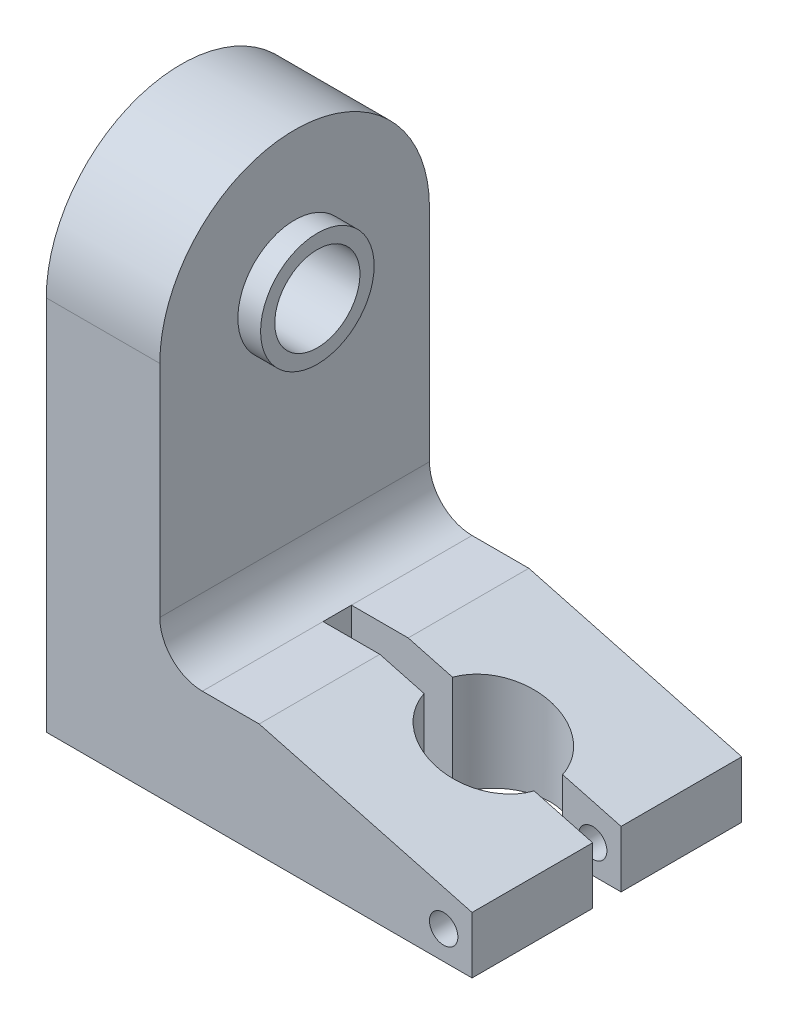
ISO-10303-21;
HEADER;
FILE_DESCRIPTION(('STEP AP214'),'2;1');
FILE_NAME('part.step','',(''),(''),'','','');
FILE_SCHEMA(('AUTOMOTIVE_DESIGN { 1 0 10303 214 1 1 1 1 }'));
ENDSEC;
DATA;
#1=APPLICATION_CONTEXT('core data for automotive mechanical design processes');
#2=APPLICATION_PROTOCOL_DEFINITION('international standard','automotive_design',2000,#1);
#3=PRODUCT_CONTEXT('',#1,'mechanical');
#4=PRODUCT('Part','Part','',(#3));
#5=PRODUCT_RELATED_PRODUCT_CATEGORY('part','',(#4));
#6=PRODUCT_DEFINITION_FORMATION('','',#4);
#7=PRODUCT_DEFINITION_CONTEXT('part definition',#1,'design');
#8=PRODUCT_DEFINITION('design','',#6,#7);
#9=PRODUCT_DEFINITION_SHAPE('','',#8);
#10=(LENGTH_UNIT() NAMED_UNIT(*) SI_UNIT(.MILLI.,.METRE.));
#11=(NAMED_UNIT(*) PLANE_ANGLE_UNIT() SI_UNIT($,.RADIAN.));
#12=(NAMED_UNIT(*) SI_UNIT($,.STERADIAN.) SOLID_ANGLE_UNIT());
#13=UNCERTAINTY_MEASURE_WITH_UNIT(LENGTH_MEASURE(1.E-05),#10,'distance_accuracy_value','');
#14=(GEOMETRIC_REPRESENTATION_CONTEXT(3) GLOBAL_UNCERTAINTY_ASSIGNED_CONTEXT((#13)) GLOBAL_UNIT_ASSIGNED_CONTEXT((#10,
#11,#12)) REPRESENTATION_CONTEXT('',''));
#15=CARTESIAN_POINT('',(0.,0.,0.));
#16=DIRECTION('',(0.,0.,1.));
#17=DIRECTION('',(1.,0.,0.));
#18=AXIS2_PLACEMENT_3D('',#15,#16,#17);
#19=CARTESIAN_POINT('',(150.,0.,47.5));
#20=DIRECTION('',(-1.,0.,0.));
#21=DIRECTION('',(0.,0.,1.));
#22=AXIS2_PLACEMENT_3D('',#19,#20,#21);
#23=PLANE('',#22);
#24=DIRECTION('',(0.,0.,-1.));
#25=VECTOR('',#24,1.);
#26=CARTESIAN_POINT('',(150.,20.,47.5));
#27=LINE('',#26,#25);
#28=CARTESIAN_POINT('',(150.,20.,-5.));
#29=VERTEX_POINT('',#28);
#30=CARTESIAN_POINT('',(150.,20.,-47.5));
#31=VERTEX_POINT('',#30);
#32=EDGE_CURVE('E168',#29,#31,#27,.T.);
#33=ORIENTED_EDGE('',*,*,#32,.F.);
#34=DIRECTION('',(0.,1.,0.));
#35=VECTOR('',#34,1.);
#36=CARTESIAN_POINT('',(150.,-25.,-5.));
#37=LINE('',#36,#35);
#38=CARTESIAN_POINT('',(150.,0.,-5.));
#39=VERTEX_POINT('',#38);
#40=EDGE_CURVE('E226',#39,#29,#37,.T.);
#41=ORIENTED_EDGE('',*,*,#40,.F.);
#42=DIRECTION('',(0.,0.,-1.));
#43=VECTOR('',#42,1.);
#44=CARTESIAN_POINT('',(150.,0.,47.5));
#45=LINE('',#44,#43);
#46=CARTESIAN_POINT('',(150.,0.,-47.5));
#47=VERTEX_POINT('',#46);
#48=EDGE_CURVE('E173',#39,#47,#45,.T.);
#49=ORIENTED_EDGE('',*,*,#48,.T.);
#50=DIRECTION('',(0.,1.,0.));
#51=VECTOR('',#50,1.);
#52=CARTESIAN_POINT('',(150.,0.,-47.5));
#53=LINE('',#52,#51);
#54=EDGE_CURVE('E149',#47,#31,#53,.T.);
#55=ORIENTED_EDGE('',*,*,#54,.T.);
#56=EDGE_LOOP('',(#33,#41,#49,#55));
#57=FACE_BOUND('',#56,.T.);
#58=ADVANCED_FACE('F39',(#57),#23,.F.);
#59=CARTESIAN_POINT('',(150.,20.,47.5));
#60=DIRECTION('',(-0.257662650560332,-0.966234939601246,0.));
#61=DIRECTION('',(0.966234939601246,-0.257662650560332,0.));
#62=AXIS2_PLACEMENT_3D('',#59,#60,#61);
#63=PLANE('',#62);
#64=CARTESIAN_POINT('',(150.,20.,47.5));
#65=VERTEX_POINT('',#64);
#66=CARTESIAN_POINT('',(150.,20.,5.));
#67=VERTEX_POINT('',#66);
#68=EDGE_CURVE('E171',#65,#67,#27,.T.);
#69=ORIENTED_EDGE('',*,*,#68,.T.);
#70=DIRECTION('',(-0.966234939601246,0.257662650560332,0.));
#71=VECTOR('',#70,1.);
#72=CARTESIAN_POINT('',(150.,20.,5.));
#73=LINE('',#72,#71);
#74=CARTESIAN_POINT('',(129.364916731037,25.5026888717234,5.));
#75=VERTEX_POINT('',#74);
#76=EDGE_CURVE('E11',#67,#75,#73,.T.);
#77=ORIENTED_EDGE('',*,*,#76,.T.);
#78=CARTESIAN_POINT('',(110.,30.6666666666667,0.));
#79=DIRECTION('',(-0.257662650560332,-0.966234939601246,0.));
#80=DIRECTION('',(-0.966234939601246,0.257662650560332,0.));
#81=AXIS2_PLACEMENT_3D('',#78,#79,#80);
#82=ELLIPSE('',#81,20.6988995950134,20.);
#83=CARTESIAN_POINT('',(90.6350832689629,35.8306444616099,5.));
#84=VERTEX_POINT('',#83);
#85=EDGE_CURVE('E48',#75,#84,#82,.T.);
#86=ORIENTED_EDGE('',*,*,#85,.T.);
#87=DIRECTION('',(-0.966234939601246,0.257662650560332,0.));
#88=VECTOR('',#87,1.);
#89=CARTESIAN_POINT('',(150.,20.,5.00000000000001));
#90=LINE('',#89,#88);
#91=CARTESIAN_POINT('',(75.,40.,5.));
#92=VERTEX_POINT('',#91);
#93=EDGE_CURVE('E196',#84,#92,#90,.T.);
#94=ORIENTED_EDGE('',*,*,#93,.T.);
#95=DIRECTION('',(0.,0.,-1.));
#96=VECTOR('',#95,1.);
#97=CARTESIAN_POINT('',(75.,40.,47.5));
#98=LINE('',#97,#96);
#99=CARTESIAN_POINT('',(75.,40.,47.5));
#100=VERTEX_POINT('',#99);
#101=EDGE_CURVE('E170',#100,#92,#98,.T.);
#102=ORIENTED_EDGE('',*,*,#101,.F.);
#103=DIRECTION('',(-0.966234939601246,0.257662650560332,0.));
#104=VECTOR('',#103,1.);
#105=CARTESIAN_POINT('',(150.,20.,47.5));
#106=LINE('',#105,#104);
#107=EDGE_CURVE('E278',#65,#100,#106,.T.);
#108=ORIENTED_EDGE('',*,*,#107,.F.);
#109=EDGE_LOOP('',(#69,#77,#86,#94,#102,#108));
#110=FACE_BOUND('',#109,.T.);
#111=ADVANCED_FACE('F195',(#110),#63,.F.);
#112=CARTESIAN_POINT('',(75.,40.,47.5));
#113=DIRECTION('',(0.,-1.,0.));
#114=DIRECTION('',(1.,0.,0.));
#115=AXIS2_PLACEMENT_3D('',#112,#113,#114);
#116=PLANE('',#115);
#117=ORIENTED_EDGE('',*,*,#101,.T.);
#118=DIRECTION('',(1.,0.,0.));
#119=VECTOR('',#118,1.);
#120=CARTESIAN_POINT('',(55.0000000000001,40.,5.));
#121=LINE('',#120,#119);
#122=CARTESIAN_POINT('',(55.0000000000001,40.,5.));
#123=VERTEX_POINT('',#122);
#124=EDGE_CURVE('E239',#123,#92,#121,.T.);
#125=ORIENTED_EDGE('',*,*,#124,.F.);
#126=DIRECTION('',(0.,0.,-1.));
#127=VECTOR('',#126,1.);
#128=CARTESIAN_POINT('',(55.0000000000001,40.,47.5));
#129=LINE('',#128,#127);
#130=CARTESIAN_POINT('',(55.0000000000001,40.,47.5));
#131=VERTEX_POINT('',#130);
#132=EDGE_CURVE('E163',#131,#123,#129,.T.);
#133=ORIENTED_EDGE('',*,*,#132,.F.);
#134=DIRECTION('',(-1.,0.,0.));
#135=VECTOR('',#134,1.);
#136=CARTESIAN_POINT('',(75.,40.,47.5));
#137=LINE('',#136,#135);
#138=EDGE_CURVE('E121',#100,#131,#137,.T.);
#139=ORIENTED_EDGE('',*,*,#138,.F.);
#140=EDGE_LOOP('',(#117,#125,#133,#139));
#141=FACE_BOUND('',#140,.T.);
#142=ADVANCED_FACE('F288',(#141),#116,.F.);
#143=CARTESIAN_POINT('',(0.,0.,47.5));
#144=DIRECTION('',(1.,0.,0.));
#145=DIRECTION('',(0.,0.,-1.));
#146=AXIS2_PLACEMENT_3D('',#143,#144,#145);
#147=PLANE('',#146);
#148=CARTESIAN_POINT('',(0.,132.5,0.));
#149=DIRECTION('',(1.,0.,0.));
#150=DIRECTION('',(0.,0.,-1.));
#151=AXIS2_PLACEMENT_3D('',#148,#149,#150);
#152=CIRCLE('',#151,15.);
#153=CARTESIAN_POINT('',(0.,132.5,-15.));
#154=VERTEX_POINT('',#153);
#155=EDGE_CURVE('E266',#154,#154,#152,.T.);
#156=ORIENTED_EDGE('',*,*,#155,.T.);
#157=EDGE_LOOP('',(#156));
#158=FACE_BOUND('',#157,.T.);
#159=DIRECTION('',(0.,-1.,0.));
#160=VECTOR('',#159,1.);
#161=CARTESIAN_POINT('',(0.,0.,-47.5));
#162=LINE('',#161,#160);
#163=CARTESIAN_POINT('',(0.,132.5,-47.5));
#164=VERTEX_POINT('',#163);
#165=CARTESIAN_POINT('',(0.,0.,-47.5));
#166=VERTEX_POINT('',#165);
#167=EDGE_CURVE('E141',#164,#166,#162,.T.);
#168=ORIENTED_EDGE('',*,*,#167,.T.);
#169=DIRECTION('',(0.,0.,-1.));
#170=VECTOR('',#169,1.);
#171=CARTESIAN_POINT('',(0.,0.,47.5));
#172=LINE('',#171,#170);
#173=CARTESIAN_POINT('',(0.,0.,47.5));
#174=VERTEX_POINT('',#173);
#175=EDGE_CURVE('E177',#174,#166,#172,.T.);
#176=ORIENTED_EDGE('',*,*,#175,.F.);
#177=DIRECTION('',(0.,-1.,0.));
#178=VECTOR('',#177,1.);
#179=CARTESIAN_POINT('',(0.,0.,47.5));
#180=LINE('',#179,#178);
#181=CARTESIAN_POINT('',(0.,132.5,47.5));
#182=VERTEX_POINT('',#181);
#183=EDGE_CURVE('E165',#182,#174,#180,.T.);
#184=ORIENTED_EDGE('',*,*,#183,.F.);
#185=CARTESIAN_POINT('',(0.,132.5,0.));
#186=DIRECTION('',(-1.,0.,0.));
#187=DIRECTION('',(0.,0.,1.));
#188=AXIS2_PLACEMENT_3D('',#185,#186,#187);
#189=CIRCLE('',#188,47.5);
#190=EDGE_CURVE('E275',#182,#164,#189,.T.);
#191=ORIENTED_EDGE('',*,*,#190,.T.);
#192=EDGE_LOOP('',(#168,#176,#184,#191));
#193=FACE_BOUND('',#192,.T.);
#194=ADVANCED_FACE('F41',(#158,#193),#147,.F.);
#195=CARTESIAN_POINT('',(0.,0.,47.5));
#196=DIRECTION('',(0.,1.,0.));
#197=DIRECTION('',(0.,0.,1.));
#198=AXIS2_PLACEMENT_3D('',#195,#196,#197);
#199=PLANE('',#198);
#200=ORIENTED_EDGE('',*,*,#48,.F.);
#201=DIRECTION('',(-1.,0.,0.));
#202=VECTOR('',#201,1.);
#203=CARTESIAN_POINT('',(0.,0.,-4.99999999999991));
#204=LINE('',#203,#202);
#205=CARTESIAN_POINT('',(129.364916731037,0.,-4.99999999999999));
#206=VERTEX_POINT('',#205);
#207=EDGE_CURVE('E260',#39,#206,#204,.T.);
#208=ORIENTED_EDGE('',*,*,#207,.T.);
#209=CARTESIAN_POINT('',(110.,0.,0.));
#210=DIRECTION('',(0.,1.,0.));
#211=DIRECTION('',(0.,0.,1.));
#212=AXIS2_PLACEMENT_3D('',#209,#210,#211);
#213=CIRCLE('',#212,20.);
#214=CARTESIAN_POINT('',(90.6350832689629,0.,-4.99999999999998));
#215=VERTEX_POINT('',#214);
#216=EDGE_CURVE('E257',#206,#215,#213,.T.);
#217=ORIENTED_EDGE('',*,*,#216,.T.);
#218=DIRECTION('',(-1.,0.,0.));
#219=VECTOR('',#218,1.);
#220=CARTESIAN_POINT('',(0.,0.,-5.00000000000002));
#221=LINE('',#220,#219);
#222=CARTESIAN_POINT('',(55.0000000000001,0.,-5.));
#223=VERTEX_POINT('',#222);
#224=EDGE_CURVE('E249',#215,#223,#221,.T.);
#225=ORIENTED_EDGE('',*,*,#224,.T.);
#226=DIRECTION('',(0.,0.,1.));
#227=VECTOR('',#226,1.);
#228=CARTESIAN_POINT('',(55.0000000000001,0.,47.5));
#229=LINE('',#228,#227);
#230=CARTESIAN_POINT('',(55.0000000000001,0.,5.));
#231=VERTEX_POINT('',#230);
#232=EDGE_CURVE('E238',#223,#231,#229,.T.);
#233=ORIENTED_EDGE('',*,*,#232,.T.);
#234=DIRECTION('',(1.,0.,0.));
#235=VECTOR('',#234,1.);
#236=CARTESIAN_POINT('',(0.,0.,4.99999999999999));
#237=LINE('',#236,#235);
#238=CARTESIAN_POINT('',(90.6350832689629,0.,5.));
#239=VERTEX_POINT('',#238);
#240=EDGE_CURVE('E253',#231,#239,#237,.T.);
#241=ORIENTED_EDGE('',*,*,#240,.T.);
#242=CARTESIAN_POINT('',(110.,0.,0.));
#243=DIRECTION('',(0.,1.,0.));
#244=DIRECTION('',(0.,0.,1.));
#245=AXIS2_PLACEMENT_3D('',#242,#243,#244);
#246=CIRCLE('',#245,20.);
#247=CARTESIAN_POINT('',(129.364916731037,0.,5.));
#248=VERTEX_POINT('',#247);
#249=EDGE_CURVE('E255',#239,#248,#246,.T.);
#250=ORIENTED_EDGE('',*,*,#249,.T.);
#251=DIRECTION('',(1.,0.,0.));
#252=VECTOR('',#251,1.);
#253=CARTESIAN_POINT('',(0.,0.,5.00000000000002));
#254=LINE('',#253,#252);
#255=CARTESIAN_POINT('',(150.,0.,5.));
#256=VERTEX_POINT('',#255);
#257=EDGE_CURVE('E224',#248,#256,#254,.T.);
#258=ORIENTED_EDGE('',*,*,#257,.T.);
#259=CARTESIAN_POINT('',(150.,0.,47.5));
#260=VERTEX_POINT('',#259);
#261=EDGE_CURVE('E175',#260,#256,#45,.T.);
#262=ORIENTED_EDGE('',*,*,#261,.F.);
#263=DIRECTION('',(1.,0.,0.));
#264=VECTOR('',#263,1.);
#265=CARTESIAN_POINT('',(0.,0.,47.5));
#266=LINE('',#265,#264);
#267=EDGE_CURVE('E102',#174,#260,#266,.T.);
#268=ORIENTED_EDGE('',*,*,#267,.F.);
#269=ORIENTED_EDGE('',*,*,#175,.T.);
#270=DIRECTION('',(1.,0.,0.));
#271=VECTOR('',#270,1.);
#272=CARTESIAN_POINT('',(0.,0.,-47.5));
#273=LINE('',#272,#271);
#274=EDGE_CURVE('E148',#166,#47,#273,.T.);
#275=ORIENTED_EDGE('',*,*,#274,.T.);
#276=EDGE_LOOP('',(#200,#208,#217,#225,#233,#241,#250,#258,#262,#268,#269,#275));
#277=FACE_BOUND('',#276,.T.);
#278=ADVANCED_FACE('F339',(#277),#199,.F.);
#279=ORIENTED_EDGE('',*,*,#261,.T.);
#280=DIRECTION('',(0.,1.,0.));
#281=VECTOR('',#280,1.);
#282=CARTESIAN_POINT('',(150.,-25.,5.));
#283=LINE('',#282,#281);
#284=EDGE_CURVE('E221',#256,#67,#283,.T.);
#285=ORIENTED_EDGE('',*,*,#284,.T.);
#286=ORIENTED_EDGE('',*,*,#68,.F.);
#287=DIRECTION('',(0.,1.,0.));
#288=VECTOR('',#287,1.);
#289=CARTESIAN_POINT('',(150.,0.,47.5));
#290=LINE('',#289,#288);
#291=EDGE_CURVE('E279',#260,#65,#290,.T.);
#292=ORIENTED_EDGE('',*,*,#291,.F.);
#293=EDGE_LOOP('',(#279,#285,#286,#292));
#294=FACE_BOUND('',#293,.T.);
#295=ADVANCED_FACE('F340',(#294),#23,.F.);
#296=CARTESIAN_POINT('',(110.,30.6666666666667,0.));
#297=DIRECTION('',(-0.257662650560332,-0.966234939601246,0.));
#298=DIRECTION('',(-0.966234939601246,0.257662650560332,0.));
#299=AXIS2_PLACEMENT_3D('',#296,#297,#298);
#300=ELLIPSE('',#299,20.6988995950134,20.);
#301=CARTESIAN_POINT('',(90.6350832689629,35.8306444616099,-4.99999999999998));
#302=VERTEX_POINT('',#301);
#303=CARTESIAN_POINT('',(129.364916731037,25.5026888717235,-4.99999999999999));
#304=VERTEX_POINT('',#303);
#305=EDGE_CURVE('E181',#302,#304,#300,.T.);
#306=ORIENTED_EDGE('',*,*,#305,.T.);
#307=DIRECTION('',(0.966234939601246,-0.257662650560332,0.));
#308=VECTOR('',#307,1.);
#309=CARTESIAN_POINT('',(150.,20.,-5.));
#310=LINE('',#309,#308);
#311=EDGE_CURVE('E186',#304,#29,#310,.T.);
#312=ORIENTED_EDGE('',*,*,#311,.T.);
#313=ORIENTED_EDGE('',*,*,#32,.T.);
#314=DIRECTION('',(-0.966234939601246,0.257662650560332,0.));
#315=VECTOR('',#314,1.);
#316=CARTESIAN_POINT('',(150.,20.,-47.5));
#317=LINE('',#316,#315);
#318=CARTESIAN_POINT('',(75.,40.,-47.5));
#319=VERTEX_POINT('',#318);
#320=EDGE_CURVE('E155',#31,#319,#317,.T.);
#321=ORIENTED_EDGE('',*,*,#320,.T.);
#322=CARTESIAN_POINT('',(75.,40.,-4.99999999999999));
#323=VERTEX_POINT('',#322);
#324=EDGE_CURVE('E167',#323,#319,#98,.T.);
#325=ORIENTED_EDGE('',*,*,#324,.F.);
#326=DIRECTION('',(0.966234939601246,-0.257662650560332,0.));
#327=VECTOR('',#326,1.);
#328=CARTESIAN_POINT('',(150.,20.,-4.99999999999996));
#329=LINE('',#328,#327);
#330=EDGE_CURVE('E244',#323,#302,#329,.T.);
#331=ORIENTED_EDGE('',*,*,#330,.T.);
#332=EDGE_LOOP('',(#306,#312,#313,#321,#325,#331));
#333=FACE_BOUND('',#332,.T.);
#334=ADVANCED_FACE('F344',(#333),#63,.F.);
#335=CARTESIAN_POINT('',(55.0000000000001,40.,-4.99999999999999));
#336=VERTEX_POINT('',#335);
#337=CARTESIAN_POINT('',(55.0000000000001,40.,-47.5));
#338=VERTEX_POINT('',#337);
#339=EDGE_CURVE('E133',#336,#338,#129,.T.);
#340=ORIENTED_EDGE('',*,*,#339,.F.);
#341=DIRECTION('',(-1.,0.,0.));
#342=VECTOR('',#341,1.);
#343=CARTESIAN_POINT('',(90.6350832689629,40.,-4.99999999999998));
#344=LINE('',#343,#342);
#345=EDGE_CURVE('E54',#323,#336,#344,.T.);
#346=ORIENTED_EDGE('',*,*,#345,.F.);
#347=ORIENTED_EDGE('',*,*,#324,.T.);
#348=DIRECTION('',(-1.,0.,0.));
#349=VECTOR('',#348,1.);
#350=CARTESIAN_POINT('',(75.,40.,-47.5));
#351=LINE('',#350,#349);
#352=EDGE_CURVE('E154',#319,#338,#351,.T.);
#353=ORIENTED_EDGE('',*,*,#352,.T.);
#354=EDGE_LOOP('',(#340,#346,#347,#353));
#355=FACE_BOUND('',#354,.T.);
#356=ADVANCED_FACE('F346',(#355),#116,.F.);
#357=CARTESIAN_POINT('',(55.,55.,47.5));
#358=DIRECTION('',(0.,0.,-1.));
#359=DIRECTION('',(-1.,0.,0.));
#360=AXIS2_PLACEMENT_3D('',#357,#358,#359);
#361=CYLINDRICAL_SURFACE('',#360,15.);
#362=CARTESIAN_POINT('',(55.,55.,-47.5));
#363=DIRECTION('',(0.,0.,-1.));
#364=DIRECTION('',(-1.,0.,0.));
#365=AXIS2_PLACEMENT_3D('',#362,#363,#364);
#366=CIRCLE('',#365,15.);
#367=CARTESIAN_POINT('',(40.,55.,-47.5));
#368=VERTEX_POINT('',#367);
#369=EDGE_CURVE('E134',#338,#368,#366,.T.);
#370=ORIENTED_EDGE('',*,*,#369,.T.);
#371=DIRECTION('',(0.,0.,-1.));
#372=VECTOR('',#371,1.);
#373=CARTESIAN_POINT('',(40.,55.,47.5));
#374=LINE('',#373,#372);
#375=CARTESIAN_POINT('',(40.,55.,47.5));
#376=VERTEX_POINT('',#375);
#377=EDGE_CURVE('E128',#376,#368,#374,.T.);
#378=ORIENTED_EDGE('',*,*,#377,.F.);
#379=CARTESIAN_POINT('',(55.,55.,47.5));
#380=DIRECTION('',(0.,0.,-1.));
#381=DIRECTION('',(-1.,0.,0.));
#382=AXIS2_PLACEMENT_3D('',#379,#380,#381);
#383=CIRCLE('',#382,15.);
#384=EDGE_CURVE('E118',#131,#376,#383,.T.);
#385=ORIENTED_EDGE('',*,*,#384,.F.);
#386=ORIENTED_EDGE('',*,*,#132,.T.);
#387=DIRECTION('',(0.,0.,1.));
#388=VECTOR('',#387,1.);
#389=CARTESIAN_POINT('',(55.0000000000001,40.,-5.));
#390=LINE('',#389,#388);
#391=EDGE_CURVE('E292',#336,#123,#390,.T.);
#392=ORIENTED_EDGE('',*,*,#391,.F.);
#393=ORIENTED_EDGE('',*,*,#339,.T.);
#394=EDGE_LOOP('',(#370,#378,#385,#386,#392,#393));
#395=FACE_BOUND('',#394,.T.);
#396=ADVANCED_FACE('F131',(#395),#361,.F.);
#397=CARTESIAN_POINT('',(40.,132.5,47.5));
#398=DIRECTION('',(-1.,0.,0.));
#399=DIRECTION('',(0.,-1.,0.));
#400=AXIS2_PLACEMENT_3D('',#397,#398,#399);
#401=PLANE('',#400);
#402=CARTESIAN_POINT('',(40.,132.5,0.));
#403=DIRECTION('',(-1.,0.,0.));
#404=DIRECTION('',(0.,-1.,0.));
#405=AXIS2_PLACEMENT_3D('',#402,#403,#404);
#406=CIRCLE('',#405,20.);
#407=CARTESIAN_POINT('',(40.,112.5,0.));
#408=VERTEX_POINT('',#407);
#409=EDGE_CURVE('E176',#408,#408,#406,.F.);
#410=ORIENTED_EDGE('',*,*,#409,.F.);
#411=EDGE_LOOP('',(#410));
#412=FACE_BOUND('',#411,.T.);
#413=DIRECTION('',(0.,1.,0.));
#414=VECTOR('',#413,1.);
#415=CARTESIAN_POINT('',(40.,132.5,-47.5));
#416=LINE('',#415,#414);
#417=CARTESIAN_POINT('',(40.,132.5,-47.5));
#418=VERTEX_POINT('',#417);
#419=EDGE_CURVE('E92',#368,#418,#416,.T.);
#420=ORIENTED_EDGE('',*,*,#419,.T.);
#421=CARTESIAN_POINT('',(40.,132.5,0.));
#422=DIRECTION('',(-1.,0.,0.));
#423=DIRECTION('',(0.,-1.,0.));
#424=AXIS2_PLACEMENT_3D('',#421,#422,#423);
#425=CIRCLE('',#424,47.5);
#426=CARTESIAN_POINT('',(40.,132.5,47.5));
#427=VERTEX_POINT('',#426);
#428=EDGE_CURVE('E137',#418,#427,#425,.F.);
#429=ORIENTED_EDGE('',*,*,#428,.T.);
#430=DIRECTION('',(0.,1.,0.));
#431=VECTOR('',#430,1.);
#432=CARTESIAN_POINT('',(40.,132.5,47.5));
#433=LINE('',#432,#431);
#434=EDGE_CURVE('E122',#376,#427,#433,.T.);
#435=ORIENTED_EDGE('',*,*,#434,.F.);
#436=ORIENTED_EDGE('',*,*,#377,.T.);
#437=EDGE_LOOP('',(#420,#429,#435,#436));
#438=FACE_BOUND('',#437,.T.);
#439=ADVANCED_FACE('F138',(#412,#438),#401,.F.);
#440=CARTESIAN_POINT('',(55.,55.,47.5));
#441=DIRECTION('',(0.,0.,-1.));
#442=DIRECTION('',(-1.,0.,0.));
#443=AXIS2_PLACEMENT_3D('',#440,#441,#442);
#444=PLANE('',#443);
#445=CARTESIAN_POINT('',(140.,10.,47.5));
#446=DIRECTION('',(0.,0.,1.));
#447=DIRECTION('',(1.,0.,0.));
#448=AXIS2_PLACEMENT_3D('',#445,#446,#447);
#449=CIRCLE('',#448,4.99999999999999);
#450=CARTESIAN_POINT('',(145.,10.,47.5));
#451=VERTEX_POINT('',#450);
#452=EDGE_CURVE('E374',#451,#451,#449,.T.);
#453=ORIENTED_EDGE('',*,*,#452,.F.);
#454=EDGE_LOOP('',(#453));
#455=FACE_BOUND('',#454,.T.);
#456=ORIENTED_EDGE('',*,*,#183,.T.);
#457=ORIENTED_EDGE('',*,*,#267,.T.);
#458=ORIENTED_EDGE('',*,*,#291,.T.);
#459=ORIENTED_EDGE('',*,*,#107,.T.);
#460=ORIENTED_EDGE('',*,*,#138,.T.);
#461=ORIENTED_EDGE('',*,*,#384,.T.);
#462=ORIENTED_EDGE('',*,*,#434,.T.);
#463=DIRECTION('',(-1.,0.,0.));
#464=VECTOR('',#463,1.);
#465=CARTESIAN_POINT('',(0.,132.5,47.5));
#466=LINE('',#465,#464);
#467=EDGE_CURVE('E63',#427,#182,#466,.T.);
#468=ORIENTED_EDGE('',*,*,#467,.T.);
#469=EDGE_LOOP('',(#456,#457,#458,#459,#460,#461,#462,#468));
#470=FACE_BOUND('',#469,.T.);
#471=ADVANCED_FACE('F123',(#455,#470),#444,.F.);
#472=CARTESIAN_POINT('',(55.,55.,-47.5));
#473=DIRECTION('',(0.,0.,-1.));
#474=DIRECTION('',(-1.,0.,0.));
#475=AXIS2_PLACEMENT_3D('',#472,#473,#474);
#476=PLANE('',#475);
#477=CARTESIAN_POINT('',(140.,10.,-47.5));
#478=DIRECTION('',(0.,0.,1.));
#479=DIRECTION('',(1.,0.,0.));
#480=AXIS2_PLACEMENT_3D('',#477,#478,#479);
#481=CIRCLE('',#480,4.99999999999999);
#482=CARTESIAN_POINT('',(145.,10.,-47.5));
#483=VERTEX_POINT('',#482);
#484=EDGE_CURVE('E378',#483,#483,#481,.T.);
#485=ORIENTED_EDGE('',*,*,#484,.T.);
#486=EDGE_LOOP('',(#485));
#487=FACE_BOUND('',#486,.T.);
#488=ORIENTED_EDGE('',*,*,#167,.F.);
#489=DIRECTION('',(-1.,0.,0.));
#490=VECTOR('',#489,1.);
#491=CARTESIAN_POINT('',(0.,132.5,-47.5));
#492=LINE('',#491,#490);
#493=EDGE_CURVE('E159',#418,#164,#492,.T.);
#494=ORIENTED_EDGE('',*,*,#493,.F.);
#495=ORIENTED_EDGE('',*,*,#419,.F.);
#496=ORIENTED_EDGE('',*,*,#369,.F.);
#497=ORIENTED_EDGE('',*,*,#352,.F.);
#498=ORIENTED_EDGE('',*,*,#320,.F.);
#499=ORIENTED_EDGE('',*,*,#54,.F.);
#500=ORIENTED_EDGE('',*,*,#274,.F.);
#501=EDGE_LOOP('',(#488,#494,#495,#496,#497,#498,#499,#500));
#502=FACE_BOUND('',#501,.T.);
#503=ADVANCED_FACE('F329',(#487,#502),#476,.T.);
#504=CARTESIAN_POINT('',(146.21322893124,132.5,0.));
#505=DIRECTION('',(-1.,0.,0.));
#506=DIRECTION('',(0.,0.,1.));
#507=AXIS2_PLACEMENT_3D('',#504,#505,#506);
#508=CYLINDRICAL_SURFACE('',#507,47.5);
#509=ORIENTED_EDGE('',*,*,#428,.F.);
#510=ORIENTED_EDGE('',*,*,#493,.T.);
#511=ORIENTED_EDGE('',*,*,#190,.F.);
#512=ORIENTED_EDGE('',*,*,#467,.F.);
#513=EDGE_LOOP('',(#509,#510,#511,#512));
#514=FACE_BOUND('',#513,.T.);
#515=ADVANCED_FACE('F336',(#514),#508,.T.);
#516=CARTESIAN_POINT('',(48.,132.5,0.));
#517=DIRECTION('',(-1.,0.,0.));
#518=DIRECTION('',(0.,-1.,0.));
#519=AXIS2_PLACEMENT_3D('',#516,#517,#518);
#520=CYLINDRICAL_SURFACE('',#519,20.);
#521=CARTESIAN_POINT('',(48.,132.5,0.));
#522=DIRECTION('',(1.,0.,0.));
#523=DIRECTION('',(0.,1.,0.));
#524=AXIS2_PLACEMENT_3D('',#521,#522,#523);
#525=CIRCLE('',#524,20.);
#526=CARTESIAN_POINT('',(48.,152.5,0.));
#527=VERTEX_POINT('',#526);
#528=EDGE_CURVE('E267',#527,#527,#525,.T.);
#529=ORIENTED_EDGE('',*,*,#528,.F.);
#530=EDGE_LOOP('',(#529));
#531=FACE_BOUND('',#530,.T.);
#532=ORIENTED_EDGE('',*,*,#409,.T.);
#533=EDGE_LOOP('',(#532));
#534=FACE_BOUND('',#533,.T.);
#535=ADVANCED_FACE('F419',(#531,#534),#520,.T.);
#536=CARTESIAN_POINT('',(48.,132.5,0.));
#537=DIRECTION('',(1.,0.,0.));
#538=DIRECTION('',(0.,1.,0.));
#539=AXIS2_PLACEMENT_3D('',#536,#537,#538);
#540=PLANE('',#539);
#541=CARTESIAN_POINT('',(48.,132.5,0.));
#542=DIRECTION('',(1.,0.,0.));
#543=DIRECTION('',(0.,1.,0.));
#544=AXIS2_PLACEMENT_3D('',#541,#542,#543);
#545=CIRCLE('',#544,15.);
#546=CARTESIAN_POINT('',(48.,147.5,0.));
#547=VERTEX_POINT('',#546);
#548=EDGE_CURVE('E263',#547,#547,#545,.T.);
#549=ORIENTED_EDGE('',*,*,#548,.F.);
#550=EDGE_LOOP('',(#549));
#551=FACE_BOUND('',#550,.T.);
#552=ORIENTED_EDGE('',*,*,#528,.T.);
#553=EDGE_LOOP('',(#552));
#554=FACE_BOUND('',#553,.T.);
#555=ADVANCED_FACE('F418',(#551,#554),#540,.T.);
#556=CARTESIAN_POINT('',(-17.,132.5,0.));
#557=DIRECTION('',(1.,0.,0.));
#558=DIRECTION('',(0.,1.,0.));
#559=AXIS2_PLACEMENT_3D('',#556,#557,#558);
#560=CYLINDRICAL_SURFACE('',#559,15.);
#561=ORIENTED_EDGE('',*,*,#548,.T.);
#562=EDGE_LOOP('',(#561));
#563=FACE_BOUND('',#562,.T.);
#564=ORIENTED_EDGE('',*,*,#155,.F.);
#565=EDGE_LOOP('',(#564));
#566=FACE_BOUND('',#565,.T.);
#567=ADVANCED_FACE('F415',(#563,#566),#560,.F.);
#568=CARTESIAN_POINT('',(110.,-25.,0.));
#569=DIRECTION('',(0.,1.,0.));
#570=DIRECTION('',(-1.,0.,0.));
#571=AXIS2_PLACEMENT_3D('',#568,#569,#570);
#572=CYLINDRICAL_SURFACE('',#571,20.);
#573=DIRECTION('',(0.,1.,0.));
#574=VECTOR('',#573,1.);
#575=CARTESIAN_POINT('',(129.364916731037,-25.,-4.99999999999999));
#576=LINE('',#575,#574);
#577=EDGE_CURVE('E243',#206,#304,#576,.T.);
#578=ORIENTED_EDGE('',*,*,#577,.T.);
#579=ORIENTED_EDGE('',*,*,#305,.F.);
#580=DIRECTION('',(0.,1.,0.));
#581=VECTOR('',#580,1.);
#582=CARTESIAN_POINT('',(90.6350832689629,-25.,-4.99999999999998));
#583=LINE('',#582,#581);
#584=EDGE_CURVE('E237',#215,#302,#583,.T.);
#585=ORIENTED_EDGE('',*,*,#584,.F.);
#586=ORIENTED_EDGE('',*,*,#216,.F.);
#587=EDGE_LOOP('',(#578,#579,#585,#586));
#588=FACE_BOUND('',#587,.T.);
#589=ADVANCED_FACE('F365',(#588),#572,.F.);
#590=CARTESIAN_POINT('',(129.364916731037,-25.,-4.99999999999999));
#591=DIRECTION('',(0.,0.,-1.));
#592=DIRECTION('',(-1.,0.,0.));
#593=AXIS2_PLACEMENT_3D('',#590,#591,#592);
#594=PLANE('',#593);
#595=CARTESIAN_POINT('',(140.,10.,-5.));
#596=DIRECTION('',(0.,0.,-1.));
#597=DIRECTION('',(-1.,0.,0.));
#598=AXIS2_PLACEMENT_3D('',#595,#596,#597);
#599=CIRCLE('',#598,4.99999999999999);
#600=CARTESIAN_POINT('',(135.,10.,-4.99999999999999));
#601=VERTEX_POINT('',#600);
#602=EDGE_CURVE('E375',#601,#601,#599,.T.);
#603=ORIENTED_EDGE('',*,*,#602,.T.);
#604=EDGE_LOOP('',(#603));
#605=FACE_BOUND('',#604,.T.);
#606=ORIENTED_EDGE('',*,*,#40,.T.);
#607=ORIENTED_EDGE('',*,*,#311,.F.);
#608=ORIENTED_EDGE('',*,*,#577,.F.);
#609=ORIENTED_EDGE('',*,*,#207,.F.);
#610=EDGE_LOOP('',(#606,#607,#608,#609));
#611=FACE_BOUND('',#610,.T.);
#612=ADVANCED_FACE('F368',(#605,#611),#594,.F.);
#613=CARTESIAN_POINT('',(129.364916731037,-25.,5.));
#614=DIRECTION('',(0.,0.,1.));
#615=DIRECTION('',(1.,0.,0.));
#616=AXIS2_PLACEMENT_3D('',#613,#614,#615);
#617=PLANE('',#616);
#618=CARTESIAN_POINT('',(140.,10.,5.));
#619=DIRECTION('',(0.,0.,1.));
#620=DIRECTION('',(1.,0.,0.));
#621=AXIS2_PLACEMENT_3D('',#618,#619,#620);
#622=CIRCLE('',#621,4.99999999999999);
#623=CARTESIAN_POINT('',(145.,10.,5.));
#624=VERTEX_POINT('',#623);
#625=EDGE_CURVE('E43',#624,#624,#622,.T.);
#626=ORIENTED_EDGE('',*,*,#625,.T.);
#627=EDGE_LOOP('',(#626));
#628=FACE_BOUND('',#627,.T.);
#629=DIRECTION('',(0.,1.,0.));
#630=VECTOR('',#629,1.);
#631=CARTESIAN_POINT('',(129.364916731037,-25.,5.));
#632=LINE('',#631,#630);
#633=EDGE_CURVE('E209',#248,#75,#632,.T.);
#634=ORIENTED_EDGE('',*,*,#633,.T.);
#635=ORIENTED_EDGE('',*,*,#76,.F.);
#636=ORIENTED_EDGE('',*,*,#284,.F.);
#637=ORIENTED_EDGE('',*,*,#257,.F.);
#638=EDGE_LOOP('',(#634,#635,#636,#637));
#639=FACE_BOUND('',#638,.T.);
#640=ADVANCED_FACE('F217',(#628,#639),#617,.F.);
#641=CARTESIAN_POINT('',(110.,-25.,0.));
#642=DIRECTION('',(0.,1.,0.));
#643=DIRECTION('',(-1.,0.,0.));
#644=AXIS2_PLACEMENT_3D('',#641,#642,#643);
#645=CYLINDRICAL_SURFACE('',#644,20.);
#646=DIRECTION('',(0.,1.,0.));
#647=VECTOR('',#646,1.);
#648=CARTESIAN_POINT('',(90.6350832689629,-25.,5.));
#649=LINE('',#648,#647);
#650=EDGE_CURVE('E213',#239,#84,#649,.T.);
#651=ORIENTED_EDGE('',*,*,#650,.T.);
#652=ORIENTED_EDGE('',*,*,#85,.F.);
#653=ORIENTED_EDGE('',*,*,#633,.F.);
#654=ORIENTED_EDGE('',*,*,#249,.F.);
#655=EDGE_LOOP('',(#651,#652,#653,#654));
#656=FACE_BOUND('',#655,.T.);
#657=ADVANCED_FACE('F208',(#656),#645,.F.);
#658=CARTESIAN_POINT('',(55.0000000000001,-25.,5.));
#659=DIRECTION('',(0.,0.,1.));
#660=DIRECTION('',(1.,0.,0.));
#661=AXIS2_PLACEMENT_3D('',#658,#659,#660);
#662=PLANE('',#661);
#663=DIRECTION('',(0.,1.,0.));
#664=VECTOR('',#663,1.);
#665=CARTESIAN_POINT('',(55.0000000000001,-25.,5.));
#666=LINE('',#665,#664);
#667=EDGE_CURVE('E229',#231,#123,#666,.T.);
#668=ORIENTED_EDGE('',*,*,#667,.T.);
#669=ORIENTED_EDGE('',*,*,#124,.T.);
#670=ORIENTED_EDGE('',*,*,#93,.F.);
#671=ORIENTED_EDGE('',*,*,#650,.F.);
#672=ORIENTED_EDGE('',*,*,#240,.F.);
#673=EDGE_LOOP('',(#668,#669,#670,#671,#672));
#674=FACE_BOUND('',#673,.T.);
#675=ADVANCED_FACE('F407',(#674),#662,.F.);
#676=CARTESIAN_POINT('',(90.6350832689629,-25.,-4.99999999999998));
#677=DIRECTION('',(0.,0.,-1.));
#678=DIRECTION('',(-1.,0.,0.));
#679=AXIS2_PLACEMENT_3D('',#676,#677,#678);
#680=PLANE('',#679);
#681=ORIENTED_EDGE('',*,*,#584,.T.);
#682=ORIENTED_EDGE('',*,*,#330,.F.);
#683=ORIENTED_EDGE('',*,*,#345,.T.);
#684=DIRECTION('',(0.,1.,0.));
#685=VECTOR('',#684,1.);
#686=CARTESIAN_POINT('',(55.0000000000001,-25.,-5.));
#687=LINE('',#686,#685);
#688=EDGE_CURVE('E235',#223,#336,#687,.T.);
#689=ORIENTED_EDGE('',*,*,#688,.F.);
#690=ORIENTED_EDGE('',*,*,#224,.F.);
#691=EDGE_LOOP('',(#681,#682,#683,#689,#690));
#692=FACE_BOUND('',#691,.T.);
#693=ADVANCED_FACE('F364',(#692),#680,.F.);
#694=CARTESIAN_POINT('',(55.0000000000001,-25.,-5.));
#695=DIRECTION('',(-1.,0.,0.));
#696=DIRECTION('',(0.,-1.,0.));
#697=AXIS2_PLACEMENT_3D('',#694,#695,#696);
#698=PLANE('',#697);
#699=ORIENTED_EDGE('',*,*,#688,.T.);
#700=ORIENTED_EDGE('',*,*,#391,.T.);
#701=ORIENTED_EDGE('',*,*,#667,.F.);
#702=ORIENTED_EDGE('',*,*,#232,.F.);
#703=EDGE_LOOP('',(#699,#700,#701,#702));
#704=FACE_BOUND('',#703,.T.);
#705=ADVANCED_FACE('F386',(#704),#698,.F.);
#706=CARTESIAN_POINT('',(140.,10.,-47.5));
#707=DIRECTION('',(0.,0.,1.));
#708=DIRECTION('',(1.,0.,0.));
#709=AXIS2_PLACEMENT_3D('',#706,#707,#708);
#710=CYLINDRICAL_SURFACE('',#709,4.99999999999999);
#711=ORIENTED_EDGE('',*,*,#452,.T.);
#712=EDGE_LOOP('',(#711));
#713=FACE_BOUND('',#712,.T.);
#714=ORIENTED_EDGE('',*,*,#625,.F.);
#715=EDGE_LOOP('',(#714));
#716=FACE_BOUND('',#715,.T.);
#717=ADVANCED_FACE('F387',(#713,#716),#710,.F.);
#718=ORIENTED_EDGE('',*,*,#484,.F.);
#719=EDGE_LOOP('',(#718));
#720=FACE_BOUND('',#719,.T.);
#721=ORIENTED_EDGE('',*,*,#602,.F.);
#722=EDGE_LOOP('',(#721));
#723=FACE_BOUND('',#722,.T.);
#724=ADVANCED_FACE('F389',(#720,#723),#710,.F.);
#725=CLOSED_SHELL('',(#58,#111,#142,#194,#278,#295,#334,#356,#396,#439,#471,#503,#515,#535,#555,
#567,#589,#612,#640,#657,#675,#693,#705,#717,#724));
#726=MANIFOLD_SOLID_BREP('B2',#725);
#727=ADVANCED_BREP_SHAPE_REPRESENTATION('',(#18,#726),#14);
#728=SHAPE_DEFINITION_REPRESENTATION(#9,#727);
ENDSEC;
END-ISO-10303-21;
